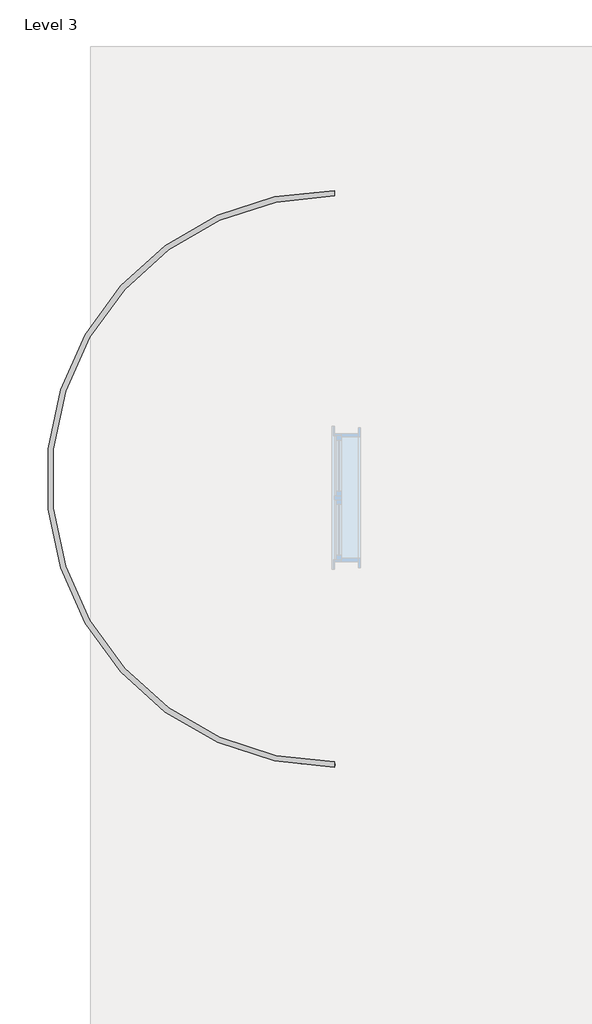
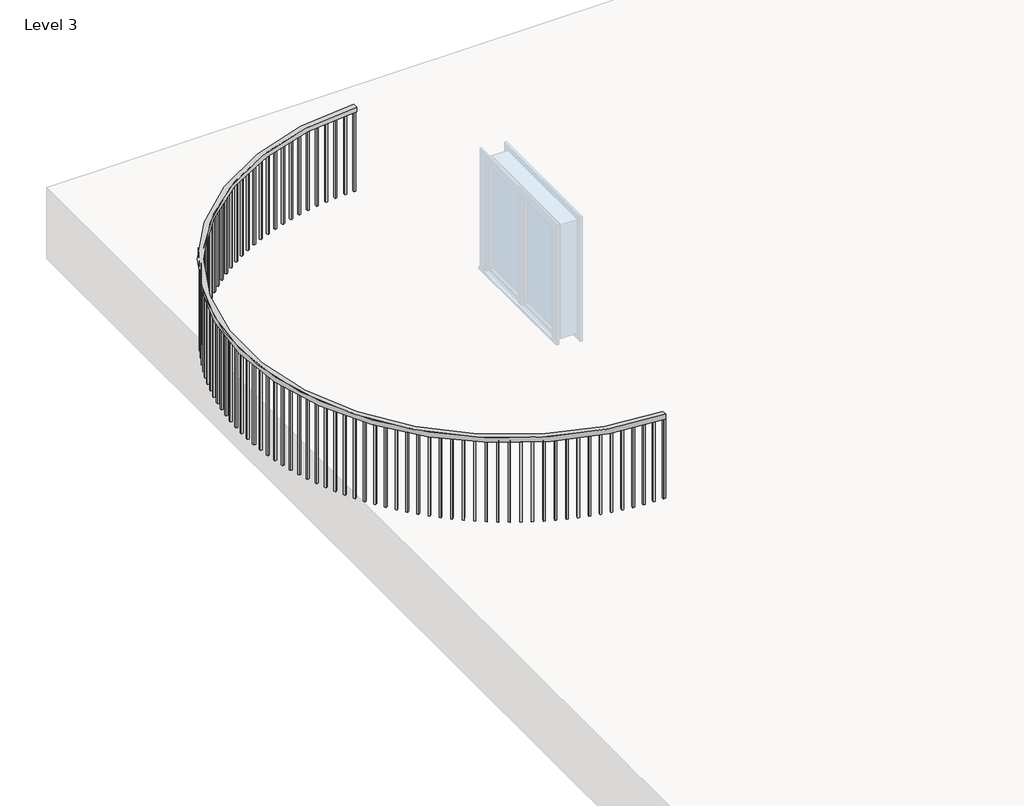
# One storey, part 2 of 2: 1 railing.
"""IFC4 building model written with IfcOpenShell, lengths in millimetres."""

from ifc_helpers import new_model, si_unit, point, frame, frame_2d, origin, place, context, project, spatial, polyline, circle_curve, trimmed, segment, composite_curve, outline, extrude, element, save

model = new_model("IFC4")

# Units and contexts
model_context = context("Model", 3, world=origin())
ifc_project = project(units=[si_unit("LENGTHUNIT", "METRE", prefix="MILLI")], contexts=[model_context])

# Site, building, storey
site = spatial("IfcSite", under=ifc_project)
building = spatial("IfcBuilding", under=site)
storey = spatial("IfcBuildingStorey", under=building, Name="Level 3", Elevation=6096.0)

# Railing
placement = place(None, origin())
element("IfcRailing", 1, ObjectType="Handrail - Rectangular", at=placement, inside=storey, context=model_context, shape_type="SweptSolid", body=[
    extrude(outline(composite_curve([segment(trimmed(circle_curve(frame_2d((-15728.6368919, 10326.9945075)), 2743.2), [point((-15728.6368919, 7583.7945075))], [point((-15728.6368919, 13070.1945075))], False, "CARTESIAN"), True, "CONTINUOUS"), segment(polyline([(-15728.6368919, 13070.1945075), (-15728.6368919, 13019.3945075)]), True, "CONTINUOUS"), segment(trimmed(circle_curve(frame_2d((-15728.6368919, 10326.9945075)), 2692.4), [point((-15728.6368919, 13019.3945075))], [point((-15728.6368919, 7634.5945075))], True, "CARTESIAN"), True, "CONTINUOUS"), segment(polyline([(-15728.6368919, 7634.5945075), (-15728.6368919, 7583.7945075)]), True, "CONTINUOUS")], self_intersect=False)), frame((0.0, 0.0, 6959.6), z_axis=(0.0, 0.0, 1.0), x_axis=(1.0, 0.0, 0.0)), (0.0, 0.0, 1.0), 50.8),
    extrude(outline(polyline([(-15741.9957848, 7599.6855919), (-15741.9690055, 7618.735573), (-15722.9190243, 7618.7087937), (-15722.9458036, 7599.6588126), (-15741.9957848, 7599.6855919)])), frame((0.0, 0.0, 6096.0), z_axis=(0.0, 0.0, 1.0), x_axis=(1.0, 0.0, 0.0)), (0.0, 0.0, 1.0), 863.6),
    extrude(outline(polyline([(-15843.9181793, 7602.0903613), (-15843.1794358, 7621.1260319), (-15824.1437651, 7620.3872884), (-15824.8825087, 7601.3516177), (-15843.9181793, 7602.0903613)])), frame((0.0, 0.0, 6096.0), z_axis=(0.0, 0.0, 1.0), x_axis=(1.0, 0.0, 0.0)), (0.0, 0.0, 1.0), 863.6),
    extrude(outline(polyline([(-15945.6794868, 7608.3027461), (-15944.2298113, 7627.297507), (-15925.2350504, 7625.8478315), (-15926.6847259, 7606.8530706), (-15945.6794868, 7608.3027461)])), frame((0.0, 0.0, 6096.0), z_axis=(0.0, 0.0, 1.0), x_axis=(1.0, 0.0, 0.0)), (0.0, 0.0, 1.0), 863.6),
    extrude(outline(polyline([(-16047.1375121, 7618.3140656), (-16044.9789303, 7637.2413746), (-16026.0516213, 7635.0827927), (-16028.2102032, 7616.1554838), (-16047.1375121, 7618.3140656)])), frame((0.0, 0.0, 6096.0), z_axis=(0.0, 0.0, 1.0), x_axis=(1.0, 0.0, 0.0)), (0.0, 0.0, 1.0), 863.6),
    extrude(outline(polyline([(-16148.150484, 7632.1103305), (-16145.2860122, 7650.9437397), (-16126.452603, 7648.0792678), (-16129.3170749, 7629.2458587), (-16148.150484, 7632.1103305)])), frame((0.0, 0.0, 6096.0), z_axis=(0.0, 0.0, 1.0), x_axis=(1.0, 0.0, 0.0)), (0.0, 0.0, 1.0), 863.6),
    extrude(outline(polyline([(-16248.5772532, 7649.6722628), (-16245.0108939, 7668.3854555), (-16226.2977012, 7664.8190963), (-16229.8640605, 7646.1059035), (-16248.5772532, 7649.6722628)])), frame((0.0, 0.0, 6096.0), z_axis=(0.0, 0.0, 1.0), x_axis=(1.0, 0.0, 0.0)), (0.0, 0.0, 1.0), 863.6),
    extrude(outline(polyline([(-16348.2774892, 7670.9753224), (-16344.014226, 7689.54215), (-16325.4473984, 7685.2788868), (-16329.7106616, 7666.7120592), (-16348.2774892, 7670.9753224)])), frame((0.0, 0.0, 6096.0), z_axis=(0.0, 0.0, 1.0), x_axis=(1.0, 0.0, 0.0)), (0.0, 0.0, 1.0), 863.6),
    extrude(outline(polyline([(-16447.1118772, 7695.9897418), (-16442.1576672, 7714.3842602), (-16423.7631489, 7709.4300502), (-16428.7173589, 7691.0355319), (-16447.1118772, 7695.9897418)])), frame((0.0, 0.0, 6096.0), z_axis=(0.0, 0.0, 1.0), x_axis=(1.0, 0.0, 0.0)), (0.0, 0.0, 1.0), 863.6),
    extrude(outline(polyline([(-16544.9423119, 7724.6805674), (-16539.3040779, 7742.8770731), (-16521.1075722, 7737.2388391), (-16526.7458062, 7719.0423334), (-16544.9423119, 7724.6805674)])), frame((0.0, 0.0, 6096.0), z_axis=(0.0, 0.0, 1.0), x_axis=(1.0, 0.0, 0.0)), (0.0, 0.0, 1.0), 863.6),
    extrude(outline(polyline([(-16641.632091, 7757.0077083), (-16635.3177115, 7774.9807746), (-16617.3446452, 7768.6663951), (-16623.6590247, 7750.6933288), (-16641.632091, 7757.0077083)])), frame((0.0, 0.0, 6096.0), z_axis=(0.0, 0.0, 1.0), x_axis=(1.0, 0.0, 0.0)), (0.0, 0.0, 1.0), 863.6),
    extrude(outline(polyline([(-16737.0461061, 7792.9259926), (-16730.0644044, 7810.6505051), (-16712.3398919, 7803.6688034), (-16719.3215936, 7785.9442909), (-16737.0461061, 7792.9259926)])), frame((0.0, 0.0, 6096.0), z_axis=(0.0, 0.0, 1.0), x_axis=(1.0, 0.0, 0.0)), (0.0, 0.0, 1.0), 863.6),
    extrude(outline(polyline([(-16831.0510314, 7832.3852302), (-16823.4117634, 7849.8364217), (-16805.9605719, 7842.1971536), (-16813.59984, 7824.7459621), (-16831.0510314, 7832.3852302)])), frame((0.0, 0.0, 6096.0), z_axis=(0.0, 0.0, 1.0), x_axis=(1.0, 0.0, 0.0)), (0.0, 0.0, 1.0), 863.6),
    extrude(outline(polyline([(-16923.5155103, 7875.3302832), (-16915.2293505, 7892.4837684), (-16898.0758652, 7884.1976086), (-16906.362025, 7867.0441234), (-16923.5155103, 7875.3302832)])), frame((0.0, 0.0, 6096.0), z_axis=(0.0, 0.0, 1.0), x_axis=(1.0, 0.0, 0.0)), (0.0, 0.0, 1.0), 863.6),
    extrude(outline(polyline([(-17014.3103383, 7921.7011427), (-17005.3888654, 7938.5329525), (-16988.5570556, 7929.6114796), (-16997.4785285, 7912.7796698), (-17014.3103383, 7921.7011427)])), frame((0.0, 0.0, 6096.0), z_axis=(0.0, 0.0, 1.0), x_axis=(1.0, 0.0, 0.0)), (0.0, 0.0, 1.0), 863.6),
    extrude(outline(polyline([(-17103.3086445, 7971.4330131), (-17093.7643247, 7987.9196276), (-17077.2777101, 7978.3753079), (-17086.8220299, 7961.8886933), (-17103.3086445, 7971.4330131)])), frame((0.0, 0.0, 6096.0), z_axis=(0.0, 0.0, 1.0), x_axis=(1.0, 0.0, 0.0)), (0.0, 0.0, 1.0), 863.6),
    extrude(outline(polyline([(-17190.3860679, 8024.4564019), (-17180.2322379, 8040.5747838), (-17164.1138559, 8030.4209539), (-17174.2676859, 8014.3025719), (-17190.3860679, 8024.4564019)])), frame((0.0, 0.0, 6096.0), z_axis=(0.0, 0.0, 1.0), x_axis=(1.0, 0.0, 0.0)), (0.0, 0.0, 1.0), 863.6),
    extrude(outline(polyline([(-17275.4209318, 8080.6972174), (-17264.67178, 8096.424844), (-17248.9441535, 8085.6756922), (-17259.6933053, 8069.9480657), (-17275.4209318, 8080.6972174)])), frame((0.0, 0.0, 6096.0), z_axis=(0.0, 0.0, 1.0), x_axis=(1.0, 0.0, 0.0)), (0.0, 0.0, 1.0), 863.6),
    extrude(outline(polyline([(-17358.2944137, 8140.0768723), (-17346.9649603, 8155.3917666), (-17331.6500661, 8144.0623132), (-17342.9795194, 8128.747419), (-17358.2944137, 8140.0768723)])), frame((0.0, 0.0, 6096.0), z_axis=(0.0, 0.0, 1.0), x_axis=(1.0, 0.0, 0.0)), (0.0, 0.0, 1.0), 863.6),
    extrude(outline(polyline([(-17438.8907113, 8202.512393), (-17426.9967874, 8217.3931549), (-17412.1160255, 8205.499231), (-17424.0099494, 8190.6184691), (-17438.8907113, 8202.512393)])), frame((0.0, 0.0, 6096.0), z_axis=(0.0, 0.0, 1.0), x_axis=(1.0, 0.0, 0.0)), (0.0, 0.0, 1.0), 863.6),
    extrude(outline(polyline([(-17517.0972041, 8267.9165359), (-17504.6554295, 8282.3423719), (-17490.2295935, 8269.9005973), (-17502.671368, 8255.4747613), (-17517.0972041, 8267.9165359)])), frame((0.0, 0.0, 6096.0), z_axis=(0.0, 0.0, 1.0), x_axis=(1.0, 0.0, 0.0)), (0.0, 0.0, 1.0), 863.6),
    extrude(outline(polyline([(-17592.8046111, 8336.1979092), (-17579.8323713, 8350.1486616), (-17565.8816189, 8337.1764217), (-17578.8538587, 8323.2256693), (-17592.8046111, 8336.1979092)])), frame((0.0, 0.0, 6096.0), z_axis=(0.0, 0.0, 1.0), x_axis=(1.0, 0.0, 0.0)), (0.0, 0.0, 1.0), 863.6),
    extrude(outline(polyline([(-17665.9071435, 8407.2611006), (-17652.422565, 8420.7172754), (-17638.9663901, 8407.2326969), (-17652.4509687, 8393.7765221), (-17665.9071435, 8407.2611006)])), frame((0.0, 0.0, 6096.0), z_axis=(0.0, 0.0, 1.0), x_axis=(1.0, 0.0, 0.0)), (0.0, 0.0, 1.0), 863.6),
    extrude(outline(polyline([(-17736.3026522, 8481.0068109), (-17722.3245775, 8493.9496053), (-17709.3817831, 8479.9715306), (-17723.3598578, 8467.0287361), (-17736.3026522, 8481.0068109)])), frame((0.0, 0.0, 6096.0), z_axis=(0.0, 0.0, 1.0), x_axis=(1.0, 0.0, 0.0)), (0.0, 0.0, 1.0), 863.6),
    extrude(outline(polyline([(-17803.8927708, 8557.3319921), (-17789.4407321, 8569.7433206), (-17777.0294035, 8555.2912819), (-17791.4814423, 8542.8799533), (-17803.8927708, 8557.3319921)])), frame((0.0, 0.0, 6096.0), z_axis=(0.0, 0.0, 1.0), x_axis=(1.0, 0.0, 0.0)), (0.0, 0.0, 1.0), 863.6),
    extrude(outline(polyline([(-17868.583053, 8636.1299922), (-17853.6772446, 8647.992512), (-17841.8147248, 8633.0867036), (-17856.7205331, 8621.2241838), (-17868.583053, 8636.1299922)])), frame((0.0, 0.0, 6096.0), z_axis=(0.0, 0.0, 1.0), x_axis=(1.0, 0.0, 0.0)), (0.0, 0.0, 1.0), 863.6),
    extrude(outline(polyline([(-17930.2831044, 8717.2907036), (-17914.9443548, 8728.5878387), (-17903.6472197, 8713.2490891), (-17918.9859693, 8701.951954), (-17930.2831044, 8717.2907036)])), frame((0.0, 0.0, 6096.0), z_axis=(0.0, 0.0, 1.0), x_axis=(1.0, 0.0, 0.0)), (0.0, 0.0, 1.0), 863.6),
    extrude(outline(polyline([(-17988.9067092, 8800.7007172), (-17973.1564519, 8811.4166817), (-17962.4404874, 8795.6664245), (-17978.1907447, 8784.9504599), (-17988.9067092, 8800.7007172)])), frame((0.0, 0.0, 6096.0), z_axis=(0.0, 0.0, 1.0), x_axis=(1.0, 0.0, 0.0)), (0.0, 0.0, 1.0), 863.6),
    extrude(outline(polyline([(-18044.3719504, 8886.2434811), (-18028.2321938, 8896.3633011), (-18018.1123738, 8880.2235446), (-18034.2521303, 8870.1037245), (-18044.3719504, 8886.2434811)])), frame((0.0, 0.0, 6096.0), z_axis=(0.0, 0.0, 1.0), x_axis=(1.0, 0.0, 0.0)), (0.0, 0.0, 1.0), 863.6),
    extrude(outline(polyline([(-18096.6013241, 8973.7994628), (-18080.094621, 8983.3089976), (-18070.5850862, 8966.8022945), (-18087.0917894, 8957.2927597), (-18096.6013241, 8973.7994628)])), frame((0.0, 0.0, 6096.0), z_axis=(0.0, 0.0, 1.0), x_axis=(1.0, 0.0, 0.0)), (0.0, 0.0, 1.0), 863.6),
    extrude(outline(polyline([(-18145.5218483, 9063.2463171), (-18128.6712641, 9072.1322785), (-18119.7853026, 9055.2816943), (-18136.6358868, 9046.3957328), (-18145.5218483, 9063.2463171)])), frame((0.0, 0.0, 6096.0), z_axis=(0.0, 0.0, 1.0), x_axis=(1.0, 0.0, 0.0)), (0.0, 0.0, 1.0), 863.6),
    extrude(outline(polyline([(-18191.0651643, 9154.4590562), (-18173.894245, 9162.7090277), (-18165.6442735, 9145.5381083), (-18182.8151929, 9137.2881369), (-18191.0651643, 9154.4590562)])), frame((0.0, 0.0, 6096.0), z_axis=(0.0, 0.0, 1.0), x_axis=(1.0, 0.0, 0.0)), (0.0, 0.0, 1.0), 863.6),
    extrude(outline(polyline([(-18233.1676328, 9247.3102252), (-18215.7003719, 9254.9126786), (-18208.0979185, 9237.4454177), (-18225.5651793, 9229.8429643), (-18233.1676328, 9247.3102252)])), frame((0.0, 0.0, 6096.0), z_axis=(0.0, 0.0, 1.0), x_axis=(1.0, 0.0, 0.0)), (0.0, 0.0, 1.0), 863.6),
    extrude(outline(polyline([(-18271.7704221, 9341.6700793), (-18254.0312274, 9348.6143915), (-18247.0869153, 9330.8751968), (-18264.82611, 9323.9308846), (-18271.7704221, 9341.6700793)])), frame((0.0, 0.0, 6096.0), z_axis=(0.0, 0.0, 1.0), x_axis=(1.0, 0.0, 0.0)), (0.0, 0.0, 1.0), 863.6),
    extrude(outline(polyline([(-18306.8195913, 9437.4067659), (-18288.8332504, 9443.6832333), (-18282.5567831, 9425.6968925), (-18300.5431239, 9419.4204251), (-18306.8195913, 9437.4067659)])), frame((0.0, 0.0, 6096.0), z_axis=(0.0, 0.0, 1.0), x_axis=(1.0, 0.0, 0.0)), (0.0, 0.0, 1.0), 863.6),
    extrude(outline(polyline([(-18338.2661646, 9534.3865084), (-18320.0578106, 9539.9863606), (-18314.4579584, 9521.7780066), (-18332.6663124, 9516.1781544), (-18338.2661646, 9534.3865084)])), frame((0.0, 0.0, 6096.0), z_axis=(0.0, 0.0, 1.0), x_axis=(1.0, 0.0, 0.0)), (0.0, 0.0, 1.0), 863.6),
    extrude(outline(polyline([(-18366.0662006, 9632.4737931), (-18347.6612768, 9637.3892053), (-18342.7458646, 9618.9842814), (-18361.1507885, 9614.0688692), (-18366.0662006, 9632.4737931)])), frame((0.0, 0.0, 6096.0), z_axis=(0.0, 0.0, 1.0), x_axis=(1.0, 0.0, 0.0)), (0.0, 0.0, 1.0), 863.6),
    extrude(outline(polyline([(-18390.1808532, 9731.5315588), (-18371.6050774, 9735.7556625), (-18367.3809737, 9717.1798866), (-18385.9567496, 9712.955783), (-18390.1808532, 9731.5315588)])), frame((0.0, 0.0, 6096.0), z_axis=(0.0, 0.0, 1.0), x_axis=(1.0, 0.0, 0.0)), (0.0, 0.0, 1.0), 863.6),
    extrude(outline(polyline([(-18410.576426, 9831.4213883), (-18391.8557549, 9834.9482809), (-18388.3288623, 9816.2276097), (-18407.0495335, 9812.7007171), (-18410.576426, 9831.4213883)])), frame((0.0, 0.0, 6096.0), z_axis=(0.0, 0.0, 1.0), x_axis=(1.0, 0.0, 0.0)), (0.0, 0.0, 1.0), 863.6),
    extrude(outline(polyline([(-18427.2244196, 9932.0037015), (-18408.3850122, 9934.8284548), (-18405.560259, 9915.9890475), (-18424.3996663, 9913.1642942), (-18427.2244196, 9932.0037015)])), frame((0.0, 0.0, 6096.0), z_axis=(0.0, 0.0, 1.0), x_axis=(1.0, 0.0, 0.0)), (0.0, 0.0, 1.0), 863.6),
    extrude(outline(polyline([(-18440.1015709, 10033.1379509), (-18421.1697524, 10035.2566177), (-18419.0510856, 10016.3247992), (-18437.9829041, 10014.2061324), (-18440.1015709, 10033.1379509)])), frame((0.0, 0.0, 6096.0), z_axis=(0.0, 0.0, 1.0), x_axis=(1.0, 0.0, 0.0)), (0.0, 0.0, 1.0), 863.6),
    extrude(outline(polyline([(-18449.1898863, 10134.6828176), (-18430.1921108, 10136.0924374), (-18428.782491, 10117.094662), (-18447.7802664, 10115.6850421), (-18449.1898863, 10134.6828176)])), frame((0.0, 0.0, 6096.0), z_axis=(0.0, 0.0, 1.0), x_axis=(1.0, 0.0, 0.0)), (0.0, 0.0, 1.0), 863.6),
    extrude(outline(polyline([(-18454.4766663, 10236.4964089), (-18435.4394802, 10237.1950121), (-18434.740877, 10218.157826), (-18453.7780631, 10217.4592228), (-18454.4766663, 10236.4964089)])), frame((0.0, 0.0, 6096.0), z_axis=(0.0, 0.0, 1.0), x_axis=(1.0, 0.0, 0.0)), (0.0, 0.0, 1.0), 863.6),
    extrude(outline(polyline([(-18455.9545234, 10338.4364568), (-18436.9045281, 10338.4230671), (-18436.9179178, 10319.3730718), (-18455.967913, 10319.3864615), (-18455.9545234, 10338.4364568)])), frame((0.0, 0.0, 6096.0), z_axis=(0.0, 0.0, 1.0), x_axis=(1.0, 0.0, 0.0)), (0.0, 0.0, 1.0), 863.6),
    extrude(outline(polyline([(-18453.6213926, 10440.3605163), (-18434.5852074, 10439.6351526), (-18435.3105712, 10420.5989673), (-18454.3467564, 10421.3243311), (-18453.6213926, 10440.3605163)])), frame((0.0, 0.0, 6096.0), z_axis=(0.0, 0.0, 1.0), x_axis=(1.0, 0.0, 0.0)), (0.0, 0.0, 1.0), 863.6),
    extrude(outline(polyline([(-18447.4805342, 10542.1261652), (-18428.4847591, 10540.6898408), (-18429.9210834, 10521.6940657), (-18448.9168585, 10523.13039), (-18447.4805342, 10542.1261652)])), frame((0.0, 0.0, 6096.0), z_axis=(0.0, 0.0, 1.0), x_axis=(1.0, 0.0, 0.0)), (0.0, 0.0, 1.0), 863.6),
    extrude(outline(polyline([(-18437.5405288, 10643.5912021), (-18418.6117074, 10641.4459242), (-18420.7569852, 10622.5171027), (-18439.6858067, 10624.6623806), (-18437.5405288, 10643.5912021)])), frame((0.0, 0.0, 6096.0), z_axis=(0.0, 0.0, 1.0), x_axis=(1.0, 0.0, 0.0)), (0.0, 0.0, 1.0), 863.6),
    extrude(outline(polyline([(-18423.8152662, 10744.613846), (-18404.9798483, 10741.7626123), (-18407.8310821, 10722.9271944), (-18426.6664999, 10725.7784281), (-18423.8152662, 10744.613846)])), frame((0.0, 0.0, 6096.0), z_axis=(0.0, 0.0, 1.0), x_axis=(1.0, 0.0, 0.0)), (0.0, 0.0, 1.0), 863.6),
    extrude(outline(polyline([(-18406.3239251, 10845.0529341), (-18387.6082304, 10841.4997286), (-18391.1614358, 10822.7840338), (-18409.8771306, 10826.3372393), (-18406.3239251, 10845.0529341)])), frame((0.0, 0.0, 6096.0), z_axis=(0.0, 0.0, 1.0), x_axis=(1.0, 0.0, 0.0)), (0.0, 0.0, 1.0), 863.6),
    extrude(outline(polyline([(-18385.0909469, 10944.7681188), (-18366.5211274, 10940.5179066), (-18370.7713395, 10921.9480871), (-18389.341159, 10926.1982992), (-18385.0909469, 10944.7681188)])), frame((0.0, 0.0, 6096.0), z_axis=(0.0, 0.0, 1.0), x_axis=(1.0, 0.0, 0.0)), (0.0, 0.0, 1.0), 863.6),
    extrude(outline(polyline([(-18360.1460013, 11043.6200641), (-18341.7480054, 11038.6787843), (-18346.6892852, 11020.2807884), (-18365.0872811, 11025.2220682), (-18360.1460013, 11043.6200641)])), frame((0.0, 0.0, 6096.0), z_axis=(0.0, 0.0, 1.0), x_axis=(1.0, 0.0, 0.0)), (0.0, 0.0, 1.0), 863.6),
    extrude(outline(polyline([(-18331.5239448, 11141.4706405), (-18313.3234807, 11135.8451977), (-18318.9489235, 11117.6447336), (-18337.1493876, 11123.2701765), (-18331.5239448, 11141.4706405)])), frame((0.0, 0.0, 6096.0), z_axis=(0.0, 0.0, 1.0), x_axis=(1.0, 0.0, 0.0)), (0.0, 0.0, 1.0), 863.6),
    extrude(outline(polyline([(-18299.2647721, 11238.1831175), (-18281.287272, 11231.8813723), (-18287.5890173, 11213.9038722), (-18305.5665173, 11220.2056175), (-18299.2647721, 11238.1831175)])), frame((0.0, 0.0, 6096.0), z_axis=(0.0, 0.0, 1.0), x_axis=(1.0, 0.0, 0.0)), (0.0, 0.0, 1.0), 863.6),
    extrude(outline(polyline([(-18263.4135602, 11333.6223549), (-18245.6841449, 11326.6531129), (-18252.6533869, 11308.9236976), (-18270.3828021, 11315.8929396), (-18263.4135602, 11333.6223549)])), frame((0.0, 0.0, 6096.0), z_axis=(0.0, 0.0, 1.0), x_axis=(1.0, 0.0, 0.0)), (0.0, 0.0, 1.0), 863.6),
    extrude(outline(polyline([(-18224.0204055, 11427.6549917), (-18206.5638489, 11420.0279914), (-18214.1908492, 11402.5714348), (-18231.6474057, 11410.1984351), (-18224.0204055, 11427.6549917)])), frame((0.0, 0.0, 6096.0), z_axis=(0.0, 0.0, 1.0), x_axis=(1.0, 0.0, 0.0)), (0.0, 0.0, 1.0), 863.6),
    extrude(outline(polyline([(-18181.1403535, 11520.1496324), (-18163.9810484, 11511.8755313), (-18172.2551495, 11494.7162262), (-18189.4144546, 11502.9903273), (-18181.1403535, 11520.1496324)])), frame((0.0, 0.0, 6096.0), z_axis=(0.0, 0.0, 1.0), x_axis=(1.0, 0.0, 0.0)), (0.0, 0.0, 1.0), 863.6),
    extrude(outline(polyline([(-18134.8333222, 11610.9770307), (-18117.995246, 11602.0673905), (-18126.9048862, 11585.2293142), (-18143.7429624, 11594.1389544), (-18134.8333222, 11610.9770307)])), frame((0.0, 0.0, 6096.0), z_axis=(0.0, 0.0, 1.0), x_axis=(1.0, 0.0, 0.0)), (0.0, 0.0, 1.0), 863.6),
    extrude(outline(polyline([(-18085.1640183, 11700.0102698), (-18068.6706994, 11690.4775403), (-18078.2034289, 11673.9842214), (-18094.6967478, 11683.5169509), (-18085.1640183, 11700.0102698)])), frame((0.0, 0.0, 6096.0), z_axis=(0.0, 0.0, 1.0), x_axis=(1.0, 0.0, 0.0)), (0.0, 0.0, 1.0), 863.6),
    extrude(outline(polyline([(-18032.2018467, 11787.1249402), (-18016.0763318, 11776.9824419), (-18026.2188302, 11760.8569271), (-18042.344345, 11770.9994254), (-18032.2018467, 11787.1249402)])), frame((0.0, 0.0, 6096.0), z_axis=(0.0, 0.0, 1.0), x_axis=(1.0, 0.0, 0.0)), (0.0, 0.0, 1.0), 863.6),
    extrude(outline(polyline([(-17976.0208133, 11872.199313), (-17960.2856354, 11861.4612184), (-17971.0237301, 11845.7260405), (-17986.758908, 11856.4641351), (-17976.0208133, 11872.199313)])), frame((0.0, 0.0, 6096.0), z_axis=(0.0, 0.0, 1.0), x_axis=(1.0, 0.0, 0.0)), (0.0, 0.0, 1.0), 863.6),
    extrude(outline(polyline([(-17916.6994223, 11955.1145106), (-17901.3765687, 11943.7958244), (-17912.6952549, 11928.4729708), (-17928.0181085, 11939.791657), (-17916.6994223, 11955.1145106)])), frame((0.0, 0.0, 6096.0), z_axis=(0.0, 0.0, 1.0), x_axis=(1.0, 0.0, 0.0)), (0.0, 0.0, 1.0), 863.6),
    extrude(outline(polyline([(-17854.3205656, 12035.7546722), (-17839.4314475, 12023.8712105), (-17851.3149093, 12008.9820924), (-17866.2040274, 12020.8655541), (-17854.3205656, 12035.7546722)])), frame((0.0, 0.0, 6096.0), z_axis=(0.0, 0.0, 1.0), x_axis=(1.0, 0.0, 0.0)), (0.0, 0.0, 1.0), 863.6),
    extrude(outline(polyline([(-17788.9714078, 12114.0071162), (-17774.5368304, 12101.5754842), (-17786.9684624, 12087.1409068), (-17801.4030399, 12099.5725388), (-17788.9714078, 12114.0071162)])), frame((0.0, 0.0, 6096.0), z_axis=(0.0, 0.0, 1.0), x_axis=(1.0, 0.0, 0.0)), (0.0, 0.0, 1.0), 863.6),
    extrude(outline(polyline([(-17720.7432638, 12189.7624974), (-17706.783397, 12176.8000663), (-17719.7458282, 12162.8401996), (-17733.7056949, 12175.8026307), (-17720.7432638, 12189.7624974)])), frame((0.0, 0.0, 6096.0), z_axis=(0.0, 0.0, 1.0), x_axis=(1.0, 0.0, 0.0)), (0.0, 0.0, 1.0), 863.6),
    extrude(outline(polyline([(-17649.7314714, 12262.9149599), (-17636.265822, 12249.4398426), (-17649.7409393, 12235.9741932), (-17663.2065887, 12249.4493105), (-17649.7314714, 12262.9149599)])), frame((0.0, 0.0, 6096.0), z_axis=(0.0, 0.0, 1.0), x_axis=(1.0, 0.0, 0.0)), (0.0, 0.0, 1.0), 863.6),
    extrude(outline(polyline([(-17576.0352582, 12333.3622847), (-17563.0826422, 12319.3933106), (-17577.0516164, 12306.4406946), (-17590.0042323, 12320.4096688), (-17576.0352582, 12333.3622847)])), frame((0.0, 0.0, 6096.0), z_axis=(0.0, 0.0, 1.0), x_axis=(1.0, 0.0, 0.0)), (0.0, 0.0, 1.0), 863.6),
    extrude(outline(polyline([(-17499.7576028, 12401.0060332), (-17487.3361194, 12386.5627216), (-17501.779431, 12374.1412382), (-17514.2009144, 12388.5845499), (-17499.7576028, 12401.0060332)])), frame((0.0, 0.0, 6096.0), z_axis=(0.0, 0.0, 1.0), x_axis=(1.0, 0.0, 0.0)), (0.0, 0.0, 1.0), 863.6),
    extrude(outline(polyline([(-17421.0050909, 12465.751684), (-17409.1320972, 12450.8542171), (-17424.0295641, 12438.9812234), (-17435.9025578, 12453.8786903), (-17421.0050909, 12465.751684)])), frame((0.0, 0.0, 6096.0), z_axis=(0.0, 0.0, 1.0), x_axis=(1.0, 0.0, 0.0)), (0.0, 0.0, 1.0), 863.6),
    extrude(outline(polyline([(-17339.8877666, 12527.5087656), (-17328.5798531, 12512.1779602), (-17343.9106585, 12500.8700467), (-17355.218572, 12516.2008521), (-17339.8877666, 12527.5087656)])), frame((0.0, 0.0, 6096.0), z_axis=(0.0, 0.0, 1.0), x_axis=(1.0, 0.0, 0.0)), (0.0, 0.0, 1.0), 863.6),
    extrude(outline(polyline([(-17256.5189783, 12586.1909822), (-17245.791946, 12570.4482607), (-17261.5346675, 12559.7212285), (-17272.2616997, 12575.46395), (-17256.5189783, 12586.1909822)])), frame((0.0, 0.0, 6096.0), z_axis=(0.0, 0.0, 1.0), x_axis=(1.0, 0.0, 0.0)), (0.0, 0.0, 1.0), 863.6),
    extrude(outline(polyline([(-17171.0152203, 12641.716335), (-17160.8840587, 12625.5836953), (-17177.0166983, 12615.4525337), (-17187.14786, 12631.5851733), (-17171.0152203, 12641.716335)])), frame((0.0, 0.0, 6096.0), z_axis=(0.0, 0.0, 1.0), x_axis=(1.0, 0.0, 0.0)), (0.0, 0.0, 1.0), 863.6),
    extrude(outline(polyline([(-17083.4959706, 12694.0072362), (-17073.9748361, 12677.5072211), (-17090.4748512, 12667.9860867), (-17099.9959857, 12684.4861018), (-17083.4959706, 12694.0072362)])), frame((0.0, 0.0, 6096.0), z_axis=(0.0, 0.0, 1.0), x_axis=(1.0, 0.0, 0.0)), (0.0, 0.0, 1.0), 863.6),
    extrude(outline(polyline([(-16994.0835232, 12742.9906177), (-16985.1857201, 12726.1462833), (-17002.0300546, 12717.2484803), (-17010.9278576, 12734.0928147), (-16994.0835232, 12742.9906177)])), frame((0.0, 0.0, 6096.0), z_axis=(0.0, 0.0, 1.0), x_axis=(1.0, 0.0, 0.0)), (0.0, 0.0, 1.0), 863.6),
    extrude(outline(polyline([(-16902.9028175, 12788.5980331), (-16894.6407792, 12771.4329166), (-16911.8058957, 12763.1708783), (-16920.067934, 12780.3359948), (-16902.9028175, 12788.5980331)])), frame((0.0, 0.0, 6096.0), z_axis=(0.0, 0.0, 1.0), x_axis=(1.0, 0.0, 0.0)), (0.0, 0.0, 1.0), 863.6),
    extrude(outline(polyline([(-16810.081264, 12830.7657533), (-16802.4665353, 12813.3038403), (-16819.9284483, 12805.6891115), (-16827.543177, 12823.1510246), (-16810.081264, 12830.7657533)])), frame((0.0, 0.0, 6096.0), z_axis=(0.0, 0.0, 1.0), x_axis=(1.0, 0.0, 0.0)), (0.0, 0.0, 1.0), 863.6),
    extrude(outline(polyline([(-16715.7485659, 12869.4348557), (-16708.7917871, 12851.7005464), (-16726.5260965, 12844.7437676), (-16733.4828752, 12862.4780769), (-16715.7485659, 12869.4348557)])), frame((0.0, 0.0, 6096.0), z_axis=(0.0, 0.0, 1.0), x_axis=(1.0, 0.0, 0.0)), (0.0, 0.0, 1.0), 863.6),
    extrude(outline(polyline([(-16620.0365379, 12904.5513065), (-16613.74743, 12886.5693817), (-16631.7293549, 12880.2802738), (-16638.0184627, 12898.2621987), (-16620.0365379, 12904.5513065)])), frame((0.0, 0.0, 6096.0), z_axis=(0.0, 0.0, 1.0), x_axis=(1.0, 0.0, 0.0)), (0.0, 0.0, 1.0), 863.6),
    extrude(outline(polyline([(-16523.0789222, 12936.0660362), (-16517.4662733, 12917.8616226), (-16535.6706868, 12912.2489737), (-16541.2833357, 12930.4533872), (-16523.0789222, 12936.0660362)])), frame((0.0, 0.0, 6096.0), z_axis=(0.0, 0.0, 1.0), x_axis=(1.0, 0.0, 0.0)), (0.0, 0.0, 1.0), 863.6),
    extrude(outline(polyline([(-16425.0112015, 12963.9350078), (-16420.0828543, 12945.5335433), (-16438.4843187, 12940.6051961), (-16443.4126659, 12959.0066606), (-16425.0112015, 12963.9350078)])), frame((0.0, 0.0, 6096.0), z_axis=(0.0, 0.0, 1.0), x_axis=(1.0, 0.0, 0.0)), (0.0, 0.0, 1.0), 863.6),
    extrude(outline(polyline([(-16325.9704097, 12988.119279), (-16321.7332507, 12969.5464768), (-16340.306053, 12965.3093178), (-16344.5432119, 12983.8821201), (-16325.9704097, 12988.119279)])), frame((0.0, 0.0, 6096.0), z_axis=(0.0, 0.0, 1.0), x_axis=(1.0, 0.0, 0.0)), (0.0, 0.0, 1.0), 863.6),
    extrude(outline(polyline([(-16226.0949403, 13008.5850563), (-16222.5548904, 12989.8668687), (-16241.273078, 12986.3268188), (-16244.8131279, 13005.0450064), (-16226.0949403, 13008.5850563)])), frame((0.0, 0.0, 6096.0), z_axis=(0.0, 0.0, 1.0), x_axis=(1.0, 0.0, 0.0)), (0.0, 0.0, 1.0), 863.6),
    extrude(outline(polyline([(-16125.5243533, 13025.3037418), (-16122.686359, 13006.4663246), (-16141.5237763, 13003.6283304), (-16144.3617705, 13022.4657476), (-16125.5243533, 13025.3037418)])), frame((0.0, 0.0, 6096.0), z_axis=(0.0, 0.0, 1.0), x_axis=(1.0, 0.0, 0.0)), (0.0, 0.0, 1.0), 863.6),
    extrude(outline(polyline([(-16024.3991798, 13038.2519741), (-16022.2672069, 13019.3216494), (-16041.1975316, 13017.1896766), (-16043.3295045, 13036.1200012), (-16024.3991798, 13038.2519741)])), frame((0.0, 0.0, 6096.0), z_axis=(0.0, 0.0, 1.0), x_axis=(1.0, 0.0, 0.0)), (0.0, 0.0, 1.0), 863.6),
    extrude(outline(polyline([(-15922.8607261, 13047.41166), (-15921.4377537, 13028.41488), (-15940.4345336, 13026.9919075), (-15941.8575061, 13045.9886875), (-15922.8607261, 13047.41166)])), frame((0.0, 0.0, 6096.0), z_axis=(0.0, 0.0, 1.0), x_axis=(1.0, 0.0, 0.0)), (0.0, 0.0, 1.0), 863.6),
    extrude(outline(polyline([(-15821.0508759, 13052.7700002), (-15820.3388922, 13033.7333099), (-15839.3755825, 13033.0213262), (-15840.0875662, 13052.0580165), (-15821.0508759, 13052.7700002)])), frame((0.0, 0.0, 6096.0), z_axis=(0.0, 0.0, 1.0), x_axis=(1.0, 0.0, 0.0)), (0.0, 0.0, 1.0), 863.6),
    extrude(outline(polyline([(-15747.7201959, 7599.7196389), (-15747.653432, 7618.7695219), (-15728.603549, 7618.702758), (-15728.6703128, 7599.652875), (-15747.7201959, 7599.7196389)])), frame((0.0, 0.0, 6096.0), z_axis=(0.0, 0.0, 1.0), x_axis=(1.0, 0.0, 0.0)), (0.0, 0.0, 1.0), 863.6),
    extrude(outline(polyline([(-15728.6703128, 13054.3361399), (-15728.603549, 13035.2862569), (-15747.653432, 13035.219493), (-15747.7201959, 13054.2693761), (-15728.6703128, 13054.3361399)])), frame((0.0, 0.0, 6096.0), z_axis=(0.0, 0.0, 1.0), x_axis=(1.0, 0.0, 0.0)), (0.0, 0.0, 1.0), 863.6),
])

save(model, "model.ifc")

# Revit data of these elements
# Type "Handrail - Rectangular"
#   Assembly Code = "C2010400"
#   built-in parameter 1008612 = 0.0416667 (stored number, unit not read)
#   built-in parameter 1008611 = 0.0416667 (stored number, unit not read)
#   built-in parameter 1008609 = 0.333333 (stored number, unit not read)
#   built-in parameter 1008604 = 0.166667 (stored number, unit not read)
#   built-in parameter 1008603 = 0.166667 (stored number, unit not read)
#   Railing Height = 3' - 0"
#   built-in parameter 1008630 = 2
#   built-in parameter 1008610 = 2
#   built-in parameter 1008618 = Baluster - Square : 3/4"
# Element 1 (IfcRailing, "Handrail - Rectangular")
#   Phase Created = New Construction
